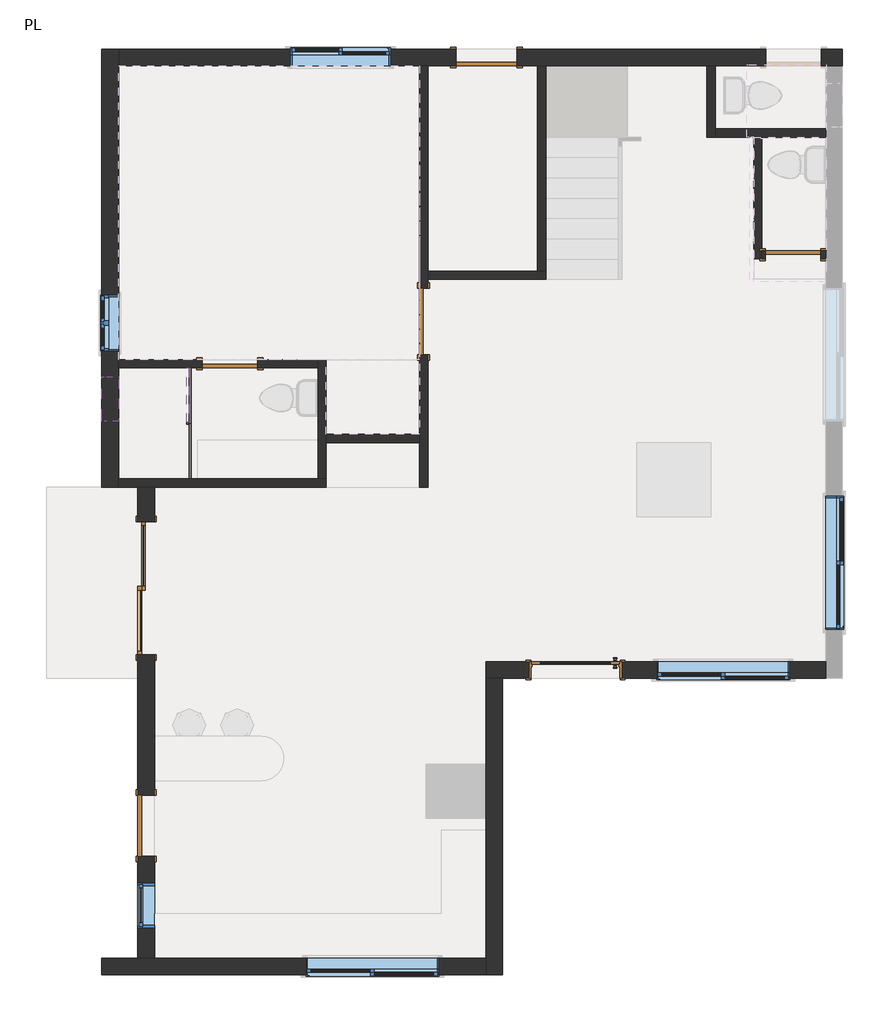
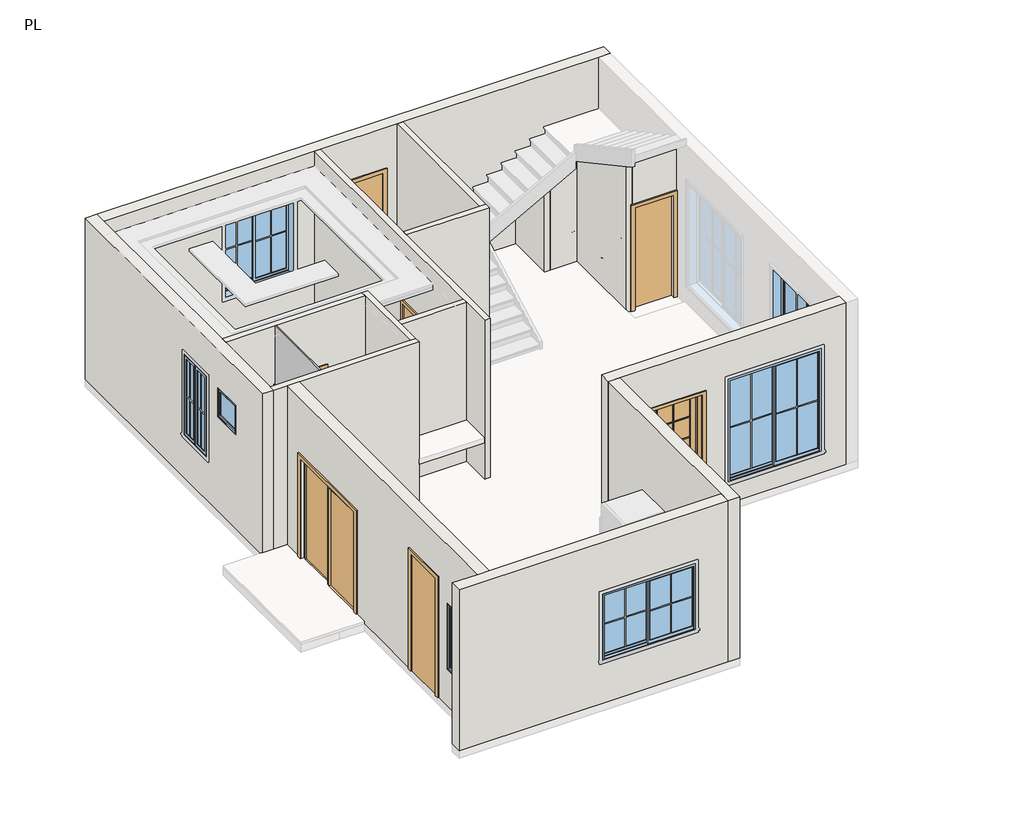
# One storey, part 1 of 2: 18 walls, 7 doors, 7 windows, 2 members, 2 plates.
"""IFC4 building model written with IfcOpenShell, lengths in millimetres."""

from ifc_helpers import new_model, si_unit, frame, origin, origin_with_axes, place, context, project, spatial, polyline, outline, extrude, faceted_brep, transform, mapped, element, save
from components import door_d4d75d1e, door_6ee39103, door_4b41b0c1, door_214872d5, door_78caadf7, door_5e62189b, member_12606fcf, member_8547658d, system_panel_glazed_13fc6ba1, system_panel_glazed_f04876f4, window_41ad1500, window_80340324, window_9dcce3b5, window_5810691a, window_sliding_double_6_x7_726fea71, window_sliding_double_6_x7_2_7e5eac46

model = new_model("IFC4")

# Units and contexts
model_context = context("Model", 3, world=origin())
ifc_project = project(units=[si_unit("LENGTHUNIT", "METRE", prefix="MILLI")], contexts=[model_context])

# Site, building, storey
site = spatial("IfcSite", under=ifc_project)
building = spatial("IfcBuilding", under=site)
storey = spatial("IfcBuildingStorey", under=building, Name="PL", Elevation=0.0)

# Doors
placement = place(None, origin())
door_shape = door_d4d75d1e(model_context)
element("IfcDoor", 1, ObjectType="Door-Double-Sliding : 72\" x 84\"", at=placement, inside=storey, context=model_context, shape_type="MappedRepresentation", body=[
    mapped(door_shape, transform((-13187.7002526, 4991.5628362, 0.0), x_axis=(0.0, 1.0, 0.0), y_axis=(-1.0, 0.0, 0.0), z_axis=(0.0, 0.0, 1.0))),
])
door_2_shape = door_6ee39103(model_context)
element("IfcDoor", 2, ObjectType="Door-Interior-Single-Full Glass-Wood : 48\" x 96\"", at=placement, inside=storey, context=model_context, shape_type="MappedRepresentation", body=[
    mapped(door_2_shape, transform((-7409.2002526, 3870.7877283, 0.0), x_axis=(-1.0, 0.0, 0.0), y_axis=(0.0, -1.0, 0.0), z_axis=(0.0, 0.0, 1.0))),
])
door_3_shape = door_4b41b0c1(model_context)
element("IfcDoor", 3, ObjectType="Single-Flush : 2'9\"X8'", at=placement, inside=storey, context=model_context, shape_type="MappedRepresentation", body=[
    mapped(door_3_shape, transform((-8634.7502526, 12287.7128362, 0.0), x_axis=(-1.0, 0.0, 0.0), y_axis=(0.0, -1.0, 0.0), z_axis=(0.0, 0.0, 1.0))),
])
element("IfcDoor", 4, ObjectType="Single-Flush : 2'9\"X8'", at=placement, inside=storey, context=model_context, shape_type="MappedRepresentation", body=[
    mapped(door_3_shape, transform((-13314.7002526, 1723.6940862, 0.0), x_axis=(0.0, 1.0, 0.0), y_axis=(-1.0, 0.0, 0.0), z_axis=(0.0, 0.0, 1.0))),
])
door_4_shape = door_214872d5(model_context)
element("IfcDoor", 5, ObjectType="Single-Flush : 30\" x 84\"", at=placement, inside=storey, context=model_context, shape_type="MappedRepresentation", body=[
    mapped(door_4_shape, transform((-4418.3502526, 9576.2628362, 0.0), x_axis=(1.0, 0.0, 0.0), y_axis=(0.0, 1.0, 0.0), z_axis=(0.0, 0.0, 1.0))),
])
door_5_shape = door_78caadf7(model_context)
element("IfcDoor", 6, ObjectType="Single-Flush : 30\" x 84\"", at=placement, inside=storey, context=model_context, shape_type="MappedRepresentation", body=[
    mapped(door_5_shape, transform((-12165.3502526, 8077.6628362, 0.0), x_axis=(1.0, 0.0, 0.0), y_axis=(0.0, 1.0, 0.0), z_axis=(0.0, 0.0, 1.0))),
])
door_6_shape = door_5e62189b(model_context)
element("IfcDoor", 7, ObjectType="Single-Flush : 36\" x 80\"", at=placement, inside=storey, context=model_context, shape_type="MappedRepresentation", body=[
    mapped(door_6_shape, transform((-9498.3502526, 8661.8628362, 0.0), x_axis=(0.0, -1.0, 0.0), y_axis=(1.0, 0.0, 0.0), z_axis=(0.0, 0.0, 1.0))),
])

# Members
member_shape = member_12606fcf(model_context)
element("IfcMember", 8, ObjectType="Rectangular Mullion : 1\" Square", at=placement, inside=storey, context=model_context, shape_type="MappedRepresentation", body=[
    mapped(member_shape, transform((-12743.285432, 7271.2128362, 2133.6), x_axis=(0.0, 0.0, 1.0), y_axis=(-1.0, 0.0, 0.0), z_axis=(0.0, -1.0, 0.0))),
])
member_2_shape = member_8547658d(model_context)
element("IfcMember", 9, ObjectType="Rectangular Mullion : 1\" Square", at=placement, inside=storey, context=model_context, shape_type="MappedRepresentation", body=[
    mapped(member_2_shape, transform((-12743.285432, 7258.5128362, 0.0), x_axis=(0.0, -1.0, 0.0), y_axis=(-1.0, 0.0, 0.0), z_axis=(0.0, 0.0, -1.0))),
])

# Plates
system_panel_glazed_shape = system_panel_glazed_13fc6ba1(model_context)
element("IfcPlate", 10, ObjectType="System Panel : Glazed", at=placement, inside=storey, context=model_context, shape_type="MappedRepresentation", body=[
    mapped(system_panel_glazed_shape, transform((-12743.285432, 7639.5128362, 0.0), x_axis=(0.0, -1.0, 0.0), y_axis=(1.0, 0.0, 0.0), z_axis=(0.0, 0.0, 1.0))),
])
system_panel_glazed_2_shape = system_panel_glazed_f04876f4(model_context)
element("IfcPlate", 11, ObjectType="System Panel : Glazed", at=placement, inside=storey, context=model_context, shape_type="MappedRepresentation", body=[
    mapped(system_panel_glazed_2_shape, transform((-12743.285432, 7258.5128362, 0.0), x_axis=(0.0, -1.0, 0.0), y_axis=(1.0, 0.0, 0.0), z_axis=(0.0, 0.0, 1.0))),
])

# Walls
element("IfcWall", 12, ObjectType="10\"", at=placement, inside=storey, context=model_context, shape_type="Brep", body=[
    faceted_brep([(-13924.3002526, 12402.0128362, 0.0), (-13924.3002526, 6382.2128362, 0.0), (-13924.3002526, 6382.2128362, 3352.8), (-13924.3002526, 12402.0128362, 3352.8), (-13924.3002526, 7899.8628362, 2565.4), (-13924.3002526, 7290.2628362, 2565.4), (-13924.3002526, 7290.2628362, 1955.8), (-13924.3002526, 7899.8628362, 1955.8), (-13924.3002526, 9017.4628362, 2590.8), (-13924.3002526, 8255.4628362, 2590.8), (-13924.3002526, 8255.4628362, 914.4), (-13924.3002526, 9017.4628362, 914.4), (-13695.7002526, 12402.0128362, 0.0), (-13695.7002526, 12402.0128362, 3352.8), (-13695.7002526, 12173.4128362, 3352.8), (-13695.7002526, 8134.8128362, 3352.8), (-13695.7002526, 8020.5128362, 3352.8), (-13695.7002526, 6496.5128362, 3352.8), (-13695.7002526, 6382.2128362, 3352.8), (-13695.7002526, 6382.2128362, 0.0), (-13695.7002526, 6496.5128362, 0.0), (-13695.7002526, 8020.5128362, 0.0), (-13695.7002526, 8134.8128362, 0.0), (-13695.7002526, 12173.4128362, 0.0), (-13695.7002526, 7899.8628362, 2565.4), (-13695.7002526, 7899.8628362, 1955.8), (-13695.7002526, 7290.2628362, 1955.8), (-13695.7002526, 7290.2628362, 2565.4), (-13695.7002526, 9017.4628362, 2590.8), (-13695.7002526, 9017.4628362, 914.4), (-13695.7002526, 8255.4628362, 914.4), (-13695.7002526, 8255.4628362, 2590.8)], [[[0, 1, 2, 3], [4, 5, 6, 7], [8, 9, 10, 11]], [[12, 13, 14, 15, 16, 17, 18, 19, 20, 21, 22, 23], [24, 25, 26, 27], [28, 29, 30, 31]], [[1, 0, 12, 23, 22, 21, 20, 19]], [[3, 2, 18, 17, 16, 15, 14, 13]], [[2, 1, 19, 18]], [[0, 3, 13, 12]], [[25, 24, 4, 7]], [[26, 25, 7, 6]], [[27, 26, 6, 5]], [[24, 27, 5, 4]], [[29, 28, 8, 11]], [[30, 29, 11, 10]], [[31, 30, 10, 9]], [[28, 31, 9, 8]]]),
])
element("IfcWall", 13, ObjectType="10\"", at=placement, inside=storey, context=model_context, shape_type="Brep", body=[
    faceted_brep([(-13695.7002526, 12173.4128362, 0.0), (-9555.5002526, 12173.4128362, 0.0), (-9441.2002526, 12173.4128362, 0.0), (-9053.8502526, 12173.4128362, 0.0), (-9053.8502526, 12173.4128362, 2438.4), (-8215.6502526, 12173.4128362, 2438.4), (-8215.6502526, 12173.4128362, 0.0), (-7929.9002526, 12173.4128362, 0.0), (-7815.6002526, 12173.4128362, 0.0), (-5599.4131221, 12173.4128362, 0.0), (-5485.1131221, 12173.4128362, 0.0), (-4793.0002526, 12173.4128362, 0.0), (-4793.0002526, 12173.4128362, 2133.6), (-4031.0002526, 12173.4128362, 2133.6), (-4031.0002526, 12173.4128362, 0.0), (-3967.5002526, 12173.4128362, 0.0), (-3738.9002526, 12173.4128362, 0.0), (-3738.9002526, 12173.4128362, 3352.8), (-3967.5002526, 12173.4128362, 3352.8), (-7815.6002526, 12173.4128362, 3352.8), (-7929.9002526, 12173.4128362, 3352.8), (-9441.2002526, 12173.4128362, 3352.8), (-9555.5002526, 12173.4128362, 3352.8), (-13695.7002526, 12173.4128362, 3352.8), (-9955.5502526, 12173.4128362, 2590.8), (-9955.5502526, 12173.4128362, 914.4), (-11327.1502526, 12173.4128362, 914.4), (-11327.1502526, 12173.4128362, 2590.8), (-9053.8502526, 12402.0128362, 2438.4), (-9053.8502526, 12402.0128362, 0.0), (-13695.7002526, 12402.0128362, 0.0), (-13695.7002526, 12402.0128362, 3352.8), (-3738.9002526, 12402.0128362, 3352.8), (-3738.9002526, 12402.0128362, 0.0), (-4031.0002526, 12402.0128362, 0.0), (-4031.0002526, 12402.0128362, 2133.6), (-4793.0002526, 12402.0128362, 2133.6), (-4793.0002526, 12402.0128362, 0.0), (-8215.6502526, 12402.0128362, 0.0), (-8215.6502526, 12402.0128362, 2438.4), (-9955.5502526, 12402.0128362, 2590.8), (-11327.1502526, 12402.0128362, 2590.8), (-11327.1502526, 12402.0128362, 914.4), (-9955.5502526, 12402.0128362, 914.4)], [[[0, 1, 2, 3, 4, 5, 6, 7, 8, 9, 10, 11, 12, 13, 14, 15, 16, 17, 18, 19, 20, 21, 22, 23], [24, 25, 26, 27]], [[28, 29, 30, 31, 32, 33, 34, 35, 36, 37, 38, 39], [40, 41, 42, 43]], [[16, 15, 14, 34, 33]], [[38, 37, 11, 10, 9, 8, 7, 6]], [[30, 29, 3, 2, 1, 0]], [[23, 22, 21, 20, 19, 18, 17, 32, 31]], [[0, 23, 31, 30]], [[17, 16, 33, 32]], [[35, 34, 14, 13]], [[36, 35, 13, 12]], [[37, 36, 12, 11]], [[4, 3, 29, 28]], [[5, 4, 28, 39]], [[6, 5, 39, 38]], [[25, 24, 40, 43]], [[26, 25, 43, 42]], [[27, 26, 42, 41]], [[24, 27, 41, 40]]]),
])
element("IfcWall", 14, ObjectType="10\"", at=placement, inside=storey, context=model_context, shape_type="Brep", body=[
    faceted_brep([(-8641.1002526, 3981.9127283, 3352.8), (-3967.5002526, 3981.9127283, 3352.8), (-3967.5002526, 3981.9127283, 0.0), (-6774.2002526, 3981.9127283, 0.0), (-6774.2002526, 3981.9127283, 2463.8), (-8044.2002526, 3981.9127283, 2463.8), (-8044.2002526, 3981.9127283, 0.0), (-8641.1002526, 3981.9127283, 0.0), (-6291.6002526, 3981.9127283, 2590.8), (-6291.6002526, 3981.9127283, 457.2), (-4462.8002526, 3981.9127283, 457.2), (-4462.8002526, 3981.9127283, 2590.8), (-3967.5002526, 3753.3127283, 3352.8), (-8412.5002526, 3753.3127283, 3352.8), (-8641.1002526, 3753.3127283, 3352.8), (-8641.1002526, 3753.3127283, 0.0), (-8412.5002526, 3753.3127283, 0.0), (-8044.2002526, 3753.3127283, 0.0), (-8044.2002526, 3753.3127283, 2463.8), (-6774.2002526, 3753.3127283, 2463.8), (-6774.2002526, 3753.3127283, 0.0), (-3967.5002526, 3753.3127283, 0.0), (-6291.6002526, 3753.3127283, 2590.8), (-4462.8002526, 3753.3127283, 2590.8), (-4462.8002526, 3753.3127283, 457.2), (-6291.6002526, 3753.3127283, 457.2)], [[[0, 1, 2, 3, 4, 5, 6, 7], [8, 9, 10, 11]], [[12, 13, 14, 15, 16, 17, 18, 19, 20, 21], [22, 23, 24, 25]], [[2, 21, 20, 3]], [[15, 7, 6, 17, 16]], [[1, 0, 14, 13, 12]], [[2, 1, 12, 21]], [[0, 7, 15, 14]], [[5, 18, 17, 6]], [[18, 5, 4, 19]], [[19, 4, 3, 20]], [[9, 8, 22, 25]], [[10, 9, 25, 24]], [[11, 10, 24, 23]], [[8, 11, 23, 22]]]),
])
element("IfcWall", 15, ObjectType="10\"", at=placement, inside=storey, context=model_context, shape_type="Brep", body=[
    faceted_brep([(-8641.1002526, 3753.3127283, 0.0), (-8641.1002526, -92.4059138, 0.0), (-8641.1002526, -321.0059138, 0.0), (-8641.1002526, -321.0059138, 3352.8), (-8641.1002526, -92.4059138, 3352.8), (-8641.1002526, 3753.3127283, 3352.8), (-8412.5002526, 3753.3127283, 0.0), (-8412.5002526, 3753.3127283, 3352.8), (-8412.5002526, -321.0059138, 3352.8), (-8412.5002526, -321.0059138, 0.0)], [[[0, 1, 2, 3, 4, 5]], [[6, 7, 8, 9]], [[2, 1, 0, 6, 9]], [[5, 4, 3, 8, 7]], [[0, 5, 7, 6]], [[3, 2, 9, 8]]]),
])
element("IfcWall", 16, ObjectType="10\"", at=placement, inside=storey, context=model_context, shape_type="Brep", body=[
    faceted_brep([(-8641.1002526, -92.4059138, 0.0), (-13200.4002526, -92.4059138, 0.0), (-13429.0002526, -92.4059138, 0.0), (-13925.8877526, -92.4059138, 0.0), (-13925.8877526, -92.4059138, 3352.8), (-13429.0002526, -92.4059138, 3352.8), (-13200.4002526, -92.4059138, 3352.8), (-8641.1002526, -92.4059138, 3352.8), (-11117.6002526, -92.4059138, 2286.0), (-11117.6002526, -92.4059138, 914.4), (-9288.8002526, -92.4059138, 914.4), (-9288.8002526, -92.4059138, 2286.0), (-8641.1002526, -321.0059138, 0.0), (-8641.1002526, -321.0059138, 3352.8), (-13925.8877526, -321.0059138, 3352.8), (-13925.8877526, -321.0059138, 0.0), (-11117.6002526, -321.0059138, 2286.0), (-9288.8002526, -321.0059138, 2286.0), (-9288.8002526, -321.0059138, 914.4), (-11117.6002526, -321.0059138, 914.4)], [[[0, 1, 2, 3, 4, 5, 6, 7], [8, 9, 10, 11]], [[12, 13, 14, 15], [16, 17, 18, 19]], [[3, 2, 1, 0, 12, 15]], [[4, 3, 15, 14]], [[7, 6, 5, 4, 14, 13]], [[0, 7, 13, 12]], [[9, 8, 16, 19]], [[10, 9, 19, 18]], [[11, 10, 18, 17]], [[8, 11, 17, 16]]]),
])
element("IfcWall", 17, ObjectType="10\"", at=placement, inside=storey, context=model_context, shape_type="SweptSolid", body=[
    extrude(outline(polyline([(4077.1628362, 0.0), (2142.7940862, 0.0), (2142.7940862, 2438.4), (1304.5940862, 2438.4), (1304.5940862, 0.0), (-92.4059138, 0.0), (-92.4059138, 3352.8), (6382.2128362, 3352.8), (6382.2128362, 0.0), (5905.9628362, 0.0), (5905.9628362, 2133.6), (4077.1628362, 2133.6), (4077.1628362, 0.0)]), holes=[polyline([(936.2940862, 2133.6), (326.6940862, 2133.6), (326.6940862, 762.0), (936.2940862, 762.0), (936.2940862, 2133.6)])]), frame((-13429.0002526, 0.0, 0.0), z_axis=(1.0, 0.0, 0.0), x_axis=(0.0, 1.0, 0.0)), (0.0, 0.0, 1.0), 228.6),
])
element("IfcWall", 18, ObjectType="5\"", at=placement, inside=storey, context=model_context, shape_type="Brep", body=[
    faceted_brep([(-13695.7002526, 6382.2128362, 0.0), (-13429.0002526, 6382.2128362, 0.0), (-13200.4002526, 6382.2128362, 0.0), (-10838.2002526, 6382.2128362, 0.0), (-10838.2002526, 6382.2128362, 3352.8), (-13200.4002526, 6382.2128362, 3352.8), (-13429.0002526, 6382.2128362, 3352.8), (-13695.7002526, 6382.2128362, 3352.8), (-13695.7002526, 6496.5128362, 0.0), (-13695.7002526, 6496.5128362, 3352.8), (-10952.5002526, 6496.5128362, 3352.8), (-10838.2002526, 6496.5128362, 3352.8), (-10838.2002526, 6496.5128362, 0.0), (-10952.5002526, 6496.5128362, 0.0)], [[[0, 1, 2, 3, 4, 5, 6, 7]], [[8, 9, 10, 11, 12, 13]], [[3, 2, 1, 0, 8, 13, 12]], [[7, 6, 5, 4, 11, 10, 9]], [[0, 7, 9, 8]], [[4, 3, 12, 11]]]),
])
element("IfcWall", 19, ObjectType="5\"", at=placement, inside=storey, context=model_context, shape_type="Brep", body=[
    faceted_brep([(-10838.2002526, 6496.5128362, 0.0), (-10838.2002526, 6991.8128362, 0.0), (-10838.2002526, 7106.1128362, 0.0), (-10838.2002526, 8134.8128362, 0.0), (-10838.2002526, 8134.8128362, 3352.8), (-10838.2002526, 7106.1128362, 3352.8), (-10838.2002526, 6991.8128362, 3352.8), (-10838.2002526, 6496.5128362, 3352.8), (-10952.5002526, 6496.5128362, 0.0), (-10952.5002526, 6496.5128362, 3352.8), (-10952.5002526, 8020.5128362, 3352.8), (-10952.5002526, 8134.8128362, 3352.8), (-10952.5002526, 8134.8128362, 0.0), (-10952.5002526, 8020.5128362, 0.0)], [[[0, 1, 2, 3, 4, 5, 6, 7]], [[8, 9, 10, 11, 12, 13]], [[3, 2, 1, 0, 8, 13, 12]], [[7, 6, 5, 4, 11, 10, 9]], [[0, 7, 9, 8]], [[4, 3, 12, 11]]]),
])
element("IfcWall", 20, ObjectType="5\"", at=placement, inside=storey, context=model_context, shape_type="SweptSolid", body=[
    extrude(outline(polyline([(2133.6, -11784.3502526), (0.0, -11784.3502526), (0.0, -10952.5002526), (3352.8, -10952.5002526), (3352.8, -13695.7002526), (0.0, -13695.7002526), (0.0, -12546.3502526), (2133.6, -12546.3502526), (2133.6, -11784.3502526)])), frame((0.0, 8020.5128362, 0.0), z_axis=(0.0, 1.0, 0.0), x_axis=(0.0, 0.0, 1.0)), (0.0, 0.0, 1.0), 114.3),
])
element("IfcWall", 21, ObjectType="5\"", at=placement, inside=storey, context=model_context, shape_type="SweptSolid", body=[
    extrude(outline(polyline([(-9555.5002526, 6991.8128362), (-10838.2002526, 6991.8128362), (-10838.2002526, 7106.1128362), (-9555.5002526, 7106.1128362), (-9555.5002526, 6991.8128362)])), origin_with_axes(), (0.0, 0.0, 1.0), 3352.8),
])
element("IfcWall", 22, ObjectType="5\"", at=placement, inside=storey, context=model_context, shape_type="Brep", body=[
    faceted_brep([(-9441.2002526, 6382.2128362, 0.0), (-9441.2002526, 8204.6628362, 0.0), (-9441.2002526, 8204.6628362, 2032.0), (-9441.2002526, 9119.0628362, 2032.0), (-9441.2002526, 9119.0628362, 0.0), (-9441.2002526, 9239.7128362, 0.0), (-9441.2002526, 9354.0128362, 0.0), (-9441.2002526, 12173.4128362, 0.0), (-9441.2002526, 12173.4128362, 3352.8), (-9441.2002526, 9354.0128362, 3352.8), (-9441.2002526, 9239.7128362, 3352.8), (-9441.2002526, 6382.2128362, 3352.8), (-9555.5002526, 8204.6628362, 2032.0), (-9555.5002526, 8204.6628362, 0.0), (-9555.5002526, 7106.1128362, 0.0), (-9555.5002526, 6991.8128362, 0.0), (-9555.5002526, 6382.2128362, 0.0), (-9555.5002526, 6382.2128362, 3352.8), (-9555.5002526, 6991.8128362, 3352.8), (-9555.5002526, 7106.1128362, 3352.8), (-9555.5002526, 12173.4128362, 3352.8), (-9555.5002526, 12173.4128362, 0.0), (-9555.5002526, 9119.0628362, 0.0), (-9555.5002526, 9119.0628362, 2032.0)], [[[0, 1, 2, 3, 4, 5, 6, 7, 8, 9, 10, 11]], [[12, 13, 14, 15, 16, 17, 18, 19, 20, 21, 22, 23]], [[22, 21, 7, 6, 5, 4]], [[16, 15, 14, 13, 1, 0]], [[11, 10, 9, 8, 20, 19, 18, 17]], [[0, 11, 17, 16]], [[8, 7, 21, 20]], [[2, 1, 13, 12]], [[3, 2, 12, 23]], [[4, 3, 23, 22]]]),
])
element("IfcWall", 23, ObjectType="5\"", at=placement, inside=storey, context=model_context, shape_type="Brep", body=[
    faceted_brep([(-9441.2002526, 9239.7128362, 0.0), (-7815.6002526, 9239.7128362, 0.0), (-7815.6002526, 9239.7128362, 3352.8), (-9441.2002526, 9239.7128362, 3352.8), (-9441.2002526, 9354.0128362, 0.0), (-9441.2002526, 9354.0128362, 3352.8), (-7929.9002526, 9354.0128362, 3352.8), (-7815.6002526, 9354.0128362, 3352.8), (-7815.6002526, 9354.0128362, 0.0), (-7929.9002526, 9354.0128362, 0.0)], [[[0, 1, 2, 3]], [[4, 5, 6, 7, 8, 9]], [[1, 0, 4, 9, 8]], [[3, 2, 7, 6, 5]], [[0, 3, 5, 4]], [[2, 1, 8, 7]]]),
])
element("IfcWall", 24, ObjectType="5\"", at=placement, inside=storey, context=model_context, shape_type="SweptSolid", body=[
    extrude(outline(polyline([(-7815.6002526, 12173.4128362), (-7815.6002526, 9354.0128362), (-7929.9002526, 9354.0128362), (-7929.9002526, 12173.4128362), (-7815.6002526, 12173.4128362)])), origin_with_axes(), (0.0, 0.0, 1.0), 3352.8),
])
element("IfcWall", 25, ObjectType="5\"", at=placement, inside=storey, context=model_context, shape_type="Brep", body=[
    faceted_brep([(-5599.4131221, 12173.4128362, 0.0), (-5599.4131221, 11195.5128362, 0.0), (-5599.4131221, 11195.5128362, 1720.85), (-5599.4131221, 12173.4128362, 1720.85), (-5485.1131221, 12173.4128362, 0.0), (-5485.1131221, 12173.4128362, 1720.85), (-5485.1131221, 11195.5128362, 1720.85), (-5485.1131221, 11195.5128362, 0.0), (-5485.1131221, 11309.8128362, 0.0)], [[[0, 1, 2, 3]], [[4, 5, 6, 7, 8]], [[0, 3, 5, 4]], [[2, 1, 7, 6]], [[1, 0, 4, 8, 7]], [[3, 2, 6, 5]]]),
])
element("IfcWall", 26, ObjectType="5\"", at=placement, inside=storey, context=model_context, shape_type="Brep", body=[
    faceted_brep([(-5485.1131221, 11195.5128362, 0.0), (-4958.1002526, 11195.5128362, 0.0), (-4843.8002526, 11195.5128362, 0.0), (-3967.5002526, 11195.5128362, 0.0), (-3967.5002526, 11195.5128362, 2057.4), (-4935.5581325, 11195.5128362, 2057.4), (-5485.1131221, 11195.5128362, 1757.642733), (-5485.1131221, 11195.5128362, 1720.85), (-5485.1131221, 11309.8128362, 0.0), (-5485.1131221, 11309.8128362, 1757.642733), (-4935.5581325, 11309.8128362, 2057.4), (-3967.5002526, 11309.8128362, 2057.4), (-3967.5002526, 11309.8128362, 0.0)], [[[0, 1, 2, 3, 4, 5, 6, 7]], [[8, 9, 10, 11, 12]], [[0, 7, 6, 9, 8]], [[4, 3, 12, 11]], [[3, 2, 1, 0, 8, 12]], [[5, 4, 11, 10]], [[6, 5, 10, 9]]]),
])
element("IfcWall", 27, ObjectType="5\"", at=placement, inside=storey, context=model_context, shape_type="Brep", body=[
    faceted_brep([(-4958.1002526, 11195.5128362, 0.0), (-4958.1002526, 9519.1128362, 0.0), (-4958.1002526, 9519.1128362, 3059.9497528), (-4958.1002526, 11195.5128362, 2145.5497528), (-4843.8002526, 11195.5128362, 0.0), (-4843.8002526, 11195.5128362, 2145.5497528), (-4843.8002526, 9519.1128362, 3059.9497528), (-4843.8002526, 9519.1128362, 0.0), (-4843.8002526, 9633.4128362, 0.0)], [[[0, 1, 2, 3]], [[4, 5, 6, 7, 8]], [[0, 3, 5, 4]], [[2, 1, 7, 6]], [[1, 0, 4, 8, 7]], [[3, 2, 6, 5]]]),
])
element("IfcWall", 28, ObjectType="5\"", at=placement, inside=storey, context=model_context, shape_type="Brep", body=[
    faceted_brep([(-4037.3502526, 9519.1128362, 2133.6), (-4037.3502526, 9519.1128362, 0.0), (-3967.5002526, 9519.1128362, 0.0), (-3967.5002526, 9519.1128362, 3149.6), (-4843.8002526, 9519.1128362, 3149.6), (-4843.8002526, 9519.1128362, 3059.9497528), (-4843.8002526, 9519.1128362, 0.0), (-4799.3502526, 9519.1128362, 0.0), (-4799.3502526, 9519.1128362, 2133.6), (-3967.5002526, 9633.4128362, 0.0), (-4037.3502526, 9633.4128362, 0.0), (-4037.3502526, 9633.4128362, 2133.6), (-4799.3502526, 9633.4128362, 2133.6), (-4799.3502526, 9633.4128362, 0.0), (-4843.8002526, 9633.4128362, 0.0), (-4843.8002526, 9633.4128362, 3149.6), (-3967.5002526, 9633.4128362, 3149.6)], [[[0, 1, 2, 3, 4, 5, 6, 7, 8]], [[9, 10, 11, 12, 13, 14, 15, 16]], [[7, 6, 14, 13]], [[2, 1, 10, 9]], [[4, 3, 16, 15]], [[6, 5, 4, 15, 14]], [[3, 2, 9, 16]], [[11, 10, 1, 0]], [[12, 11, 0, 8]], [[13, 12, 8, 7]]]),
])
element("IfcWall", 29, ObjectType="5\"", at=placement, inside=storey, context=model_context, shape_type="SweptSolid", body=[
    extrude(outline(polyline([(-11841.5002526, 2345.9940862), (-11841.5002526, 2955.5940862), (-11727.2002526, 2955.5940862), (-11727.2002526, 2345.9940862), (-11841.5002526, 2345.9940862)])), origin_with_axes(), (0.0, 0.0, 1.0), 914.4),
])

# Windows
window_shape = window_41ad1500(model_context)
element("IfcWindow", 30, ObjectType="Fixed : 2'-0\" X 4'-6\"", at=placement, inside=storey, context=model_context, shape_type="MappedRepresentation", body=[
    mapped(window_shape, transform((-13314.7002526, 669.5940862, 0.0), x_axis=(0.0, 1.0, 0.0), y_axis=(-1.0, 0.0, 0.0), z_axis=(0.0, 0.0, 1.0))),
])
window_2_shape = window_80340324(model_context)
element("IfcWindow", 31, ObjectType="Fixed : 24\" x 24\"", at=placement, inside=storey, context=model_context, shape_type="MappedRepresentation", body=[
    mapped(window_2_shape, transform((-13810.0002526, 7633.1628362, 1041.4), x_axis=(0.0, 1.0, 0.0), y_axis=(-1.0, 0.0, 0.0), z_axis=(0.0, 0.0, 1.0))),
])
window_3_shape = window_9dcce3b5(model_context)
element("IfcWindow", 32, ObjectType="Window-Casement-Double : 2'-6\" X 5'-6\"", at=placement, inside=storey, context=model_context, shape_type="MappedRepresentation", body=[
    mapped(window_3_shape, transform((-13810.0002526, 8636.4628362, 0.0), x_axis=(0.0, 1.0, 0.0), y_axis=(-1.0, 0.0, 0.0), z_axis=(0.0, 0.0, 1.0))),
])
window_4_shape = window_5810691a(model_context)
element("IfcWindow", 33, ObjectType="Window-Sliding-Double : 54\" x 66\"", at=placement, inside=storey, context=model_context, shape_type="MappedRepresentation", body=[
    mapped(window_4_shape, transform((-10641.3502526, 12291.5228362, 0.0), x_axis=(1.0, 0.0, 0.0), y_axis=(0.0, 1.0, 0.0), z_axis=(0.0, 0.0, 1.0))),
])
window_sliding_double_6_x7_shape = window_sliding_double_6_x7_726fea71(model_context)
element("IfcWindow", 34, ObjectType="Window-Sliding-Double : 6'X7'", at=placement, inside=storey, context=model_context, shape_type="MappedRepresentation", body=[
    mapped(window_sliding_double_6_x7_shape, transform((-3849.3902526, 5340.8127283, -457.2), x_axis=(0.0, -1.0, 0.0), y_axis=(1.0, 0.0, 0.0), z_axis=(0.0, 0.0, 1.0))),
])
element("IfcWindow", 35, ObjectType="Window-Sliding-Double : 6'X7'", at=placement, inside=storey, context=model_context, shape_type="MappedRepresentation", body=[
    mapped(window_sliding_double_6_x7_shape, transform((-5377.2002526, 3863.8027283, -457.2), x_axis=(-1.0, 0.0, 0.0), y_axis=(0.0, -1.0, 0.0), z_axis=(0.0, 0.0, 1.0))),
])
window_sliding_double_6_x7_2_shape = window_sliding_double_6_x7_2_7e5eac46(model_context)
element("IfcWindow", 36, ObjectType="Window-Sliding-Double : 6'X7' 2", at=placement, inside=storey, context=model_context, shape_type="MappedRepresentation", body=[
    mapped(window_sliding_double_6_x7_2_shape, transform((-10203.2002526, -210.5159138, 0.0), x_axis=(-1.0, 0.0, 0.0), y_axis=(0.0, -1.0, 0.0), z_axis=(0.0, 0.0, 1.0))),
])

save(model, "model.ifc")

# Revit data of these elements
# Type "Door-Double-Sliding : 72\" x 84\""
#   Type Mark = "10"
#   Construction Type Id = "opn-d45"
#   Assembly Code = "C1020"
#   Analytic Construction = "Wood frame, double glass door "
#   Thickness = 0' - 2"
#   Thermal Resistance (R) = 1.8150 (h·ft²·°F)/BTU
#   Heat Transfer Coefficient (U) = 0.5510 BTU/(h·ft²·°F)
#   Height = 7' - 0"
#   Rail Width = 0' - 2"
#   Stiles = 0' - 2"
#   Trim Projection Ext = 0' - 1"
#   Trim Projection Int = 0' - 1"
#   Trim Width = 0' - 3"
#   Width = 6' - 0"
#   Define Thermal Properties by = 1
#   Glazing = Glass
#   Panel Material = Wood - Birch - Solid Stained Light Low Gloss
#   Trim Material = Paint - Sienna
#   Visual Light Transmittance = 0
#   Solar Heat Gain Coefficient = 0
#   Function = (empty or 0)
#   Wall Closure = (empty or 0)
# Type "Door-Interior-Single-Full Glass-Wood : 48\" x 96\""
#   Type Mark = "8"
#   Assembly Code = "C1020300"
#   Analytic Construction = "Wood frame with single clear glass"
#   Top Rail = 0' - 4 11/16"
#   Thickness = 0' - 1 3/8"
#   Thermal Resistance (R) = 1.0102 (h·ft²·°F)/BTU
#   Swing Angle [instance default] = 90.00°
#   Stiles = 0' - 4 3/4"
#   Rough Width = 4' - 2"
#   Rough Height = 8' - 1"
#   Height = 8' - 0"
#   Width = 4' - 0"
#   Heat Transfer Coefficient (U) = 0.9900 BTU/(h·ft²·°F)
#   Bottom Rail = 0' - 9 1/8"
#   Show Grill [instance default] = yes
#   Trim Material = Cherry
#   Panel Material = Cherry
#   Frame Material = Cherry
#   Door Handle Material = Aluminum
#   Visual Light Transmittance = 0
#   Solar Heat Gain Coefficient = 0
#   Wall Closure = (empty or 0)
#   Function = (empty or 0)
# Type "Single-Flush : 2'9\"X8'"
#   Type Mark = "9"
#   Construction Type Id = "MDOOR"
#   Assembly Code = "C1020"
#   Analytic Construction = "Metal"
#   Thickness = 0' - 2"
#   Heat Transfer Coefficient (U) = 0.651978 BTU/(h·ft²·°F)
#   Height = 8' - 0"
#   Trim Projection Ext = 0' - 1"
#   Trim Projection Int = 0' - 1"
#   Trim Width = 0' - 3"
#   Width = 2' - 9"
#   Define Thermal Properties by = 1
#   Door Material = Door - Panel
#   Frame Material = Door - Frame
#   Visual Light Transmittance = 0
#   Solar Heat Gain Coefficient = 0
#   Function = (empty or 0)
#   Wall Closure = (empty or 0)
# Type "Single-Flush : 30\" x 84\""
#   Type Mark = "4"
#   Construction Type Id = "MDOOR"
#   Assembly Code = "C1020"
#   Analytic Construction = "Metal"
#   Thickness = 0' - 2"
#   Heat Transfer Coefficient (U) = 0.651978 BTU/(h·ft²·°F)
#   Height = 7' - 0"
#   Trim Projection Ext = 0' - 1"
#   Trim Projection Int = 0' - 1"
#   Trim Width = 0' - 3"
#   Width = 2' - 6"
#   Define Thermal Properties by = 1
#   Define Thermal Properties by = 1
#   Door Material = Door - Panel
#   Frame Material = Door - Frame
#   Visual Light Transmittance = 0
#   Solar Heat Gain Coefficient = 0
#   Function = (empty or 0)
#   Wall Closure = (empty or 0)
# Type "Single-Flush : 36\" x 80\""
#   Type Mark = "6"
#   Construction Type Id = "MDOOR"
#   Assembly Code = "C1020"
#   Analytic Construction = "Metal"
#   Thickness = 0' - 2"
#   Heat Transfer Coefficient (U) = 0.651978 BTU/(h·ft²·°F)
#   Height = 6' - 8"
#   Trim Projection Ext = 0' - 1"
#   Trim Projection Int = 0' - 1"
#   Trim Width = 0' - 3"
#   Width = 3' - 0"
#   Define Thermal Properties by = 1
#   Define Thermal Properties by = 1
#   Door Material = Door - Panel
#   Frame Material = Door - Frame
#   Visual Light Transmittance = 0
#   Solar Heat Gain Coefficient = 0
#   Function = (empty or 0)
#   Wall Closure = (empty or 0)
# Type "Rectangular Mullion : 1\" Square"
#   built-in parameter 1007304 = 0.0833333 (stored number, unit not read)
#   built-in parameter 1007301 = 0.0416667 (stored number, unit not read)
#   built-in parameter 1007300 = 0.0416667 (stored number, unit not read)
# Type "System Panel : Glazed"
#   Construction Type Id = "GSP4R"
#   Analytic Construction = "1/8 in Pilkington single glazing"
#   Visual Light Transmittance = 0.9
#   Solar Heat Gain Coefficient = 0.86
#   Heat Transfer Coefficient (U) = 1.18115 BTU/(h·ft²·°F)
#   Define Thermal Properties by = 1
# Type "10\""
#   Assembly Code = "B2010"
#   Layers, outside or top first: 0' - 9" "Gypsum Wall Board" (function 1)
# Type "5\""
#   Assembly Code = "B2010"
#   Layers, outside or top first: 0' - 4 1/2" "Gypsum Wall Board" (function 1)
# Type "Fixed : 2'-0\" X 4'-6\""
#   Type Mark = "22"
#   Construction Type Id = "GSP4R"
#   Assembly Code = "B2020100"
#   Analytic Construction = "1/8 in Pilkington single glazing"
#   Visual Light Transmittance = 0.9
#   Solar Heat Gain Coefficient = 0.78
#   Heat Transfer Coefficient (U) = 0.6496 BTU/(h·ft²·°F)
#   Height = 4' - 6"
#   Default Sill Height = 2' - 6"
#   Width = 2' - 0"
#   Window Inset = 0' - 0 3/4"
#   Define Thermal Properties by = 1
#   Glass Pane Material = Glass
#   Sash Material = Sash
#   Wall Closure = (empty or 0)
# Type "Fixed : 24\" x 24\""
#   Type Mark = "3"
#   Construction Type Id = "GSP4R"
#   Assembly Code = "B2020100"
#   Analytic Construction = "1/8 in Pilkington single glazing"
#   Visual Light Transmittance = 0.9
#   Solar Heat Gain Coefficient = 0.78
#   Heat Transfer Coefficient (U) = 0.6496 BTU/(h·ft²·°F)
#   Height = 2' - 0"
#   Default Sill Height = 3' - 0"
#   Width = 2' - 0"
#   Window Inset = 0' - 0 3/4"
#   Define Thermal Properties by = 1
#   Define Thermal Properties by = 1
#   Glass Pane Material = Glass
#   Sash Material = Sash
#   Wall Closure = (empty or 0)
# Type "Window-Casement-Double : 2'-6\" X 5'-6\""
#   Type Mark = "21"
#   Fire Rating = "0.5h"
#   Assembly Code = "B2020100"
#   Analytic Construction = "Double glazing - domestic"
#   Frame Extension [instance default] = 0' - 0 1/4"
#   Window Inset [instance default] = 0' - 0"
#   Wall Thickness [instance default] = 0' - 6"
#   Interior Wall Closure [instance default] = 0' - 2 1/4"
#   Half Width = 1' - 3"
#   Visual Light Transmittance = 0.81
#   Thermal Resistance (R) = 1.8146 (h·ft²·°F)/BTU
#   Solar Heat Gain Coefficient = 0.76
#   Rough Width = 2' - 6 1/2"
#   Rough Height = 5' - 6 1/2"
#   Height = 5' - 6"
#   Heat Transfer Coefficient (U) = 0.5511 BTU/(h·ft²·°F)
#   Exterior Wall Closure [instance default] = 0' - 1 1/4"
#   Extension Jamb [instance default] = 0' - 2 1/4"
#   Default Sill Height = 3' - 0"
#   Width = 2' - 6"
#   Muntin Visibility = yes
#   Interior Trim Visibility [instance default] = yes
#   Exterior Trim Visibility [instance default] = yes
#   Extension Jamb Visibility [instance default] = yes
#   Interior Trim Material = Wood - Stained
#   Muntin Pattern = Muntin Pattern_2x2 : Muntin Pattern_2x2
#   Interior Trim = Trim-Window-Interior-Flat : Picture Frame
#   Interior Frame Material = Wood - Stained
#   Glass Panel Material = Glass
#   Exterior Trim Material = Clad - White
#   Exterior Trim = Trim-Window-Exterior-Flat : with Sill
#   Exterior Frame Material = Clad - White
#   Wall Closure = (empty or 0)
# Type "Window-Sliding-Double : 54\" x 66\""
#   Type Mark = "20"
#   Fire Rating = "0.5h"
#   Assembly Code = "B2020100"
#   Analytic Construction = "Double glazing - domestic"
#   Window Inset [instance default] = 0' - 0"
#   Wall Thickness [instance default] = 0' - 6"
#   Visual Light Transmittance = 0.81
#   Thermal Resistance (R) = 1.8146 (h·ft²·°F)/BTU
#   Solar Heat Gain Coefficient = 0.76
#   Muntin Width = 1' - 11 5/8"
#   Muntin Height = 5' - 0 1/4"
#   Interior Wall Closure [instance default] = 0' - 2 3/4"
#   Heat Transfer Coefficient (U) = 0.5511 BTU/(h·ft²·°F)
#   Frame Extension [instance default] = 0' - 0 1/4"
#   Exterior Wall Closure [instance default] = 0' - 1 1/4"
#   Rough Width = 4' - 6 1/2"
#   Rough Height = 5' - 6 1/2"
#   Height = 5' - 6"
#   Extension Jamb [instance default] = 0' - 2 3/4"
#   Default Sill Height = 3' - 0"
#   Width = 4' - 6"
#   Interior Trim Visibility [instance default] = yes
#   Indicator Visibility [instance default] = yes
#   Exterior Trim Visibility [instance default] = yes
#   Muntin Visibility = yes
#   Extension Jamb Visibility [instance default] = yes
#   Muntin Pattern = Muntin Pattern_2x2 : Muntin Pattern_2x2
#   Interior Trim Material = Wood - Stained
#   Interior Trim = Trim-Window-Interior-Flat : Picture Frame
#   Interior Frame Material = Wood - Stained
#   Glass Panel Material = Glass
#   Exterior Trim Material = Clad - White
#   Exterior Trim = Trim-Window-Exterior-Flat : with Sill
#   Exterior Frame Material = Clad - White
#   Wall Closure = (empty or 0)
# Type "Window-Sliding-Double : 6'X7'"
#   Type Mark = "19"
#   Fire Rating = "0.5h"
#   Assembly Code = "B2020100"
#   Analytic Construction = "Double glazing - domestic"
#   Window Inset [instance default] = 0' - 0"
#   Wall Thickness [instance default] = 0' - 6"
#   Visual Light Transmittance = 0.81
#   Thermal Resistance (R) = 1.8146 (h·ft²·°F)/BTU
#   Solar Heat Gain Coefficient = 0.76
#   Muntin Width = 2' - 8 5/8"
#   Muntin Height = 6' - 6 1/4"
#   Interior Wall Closure [instance default] = 0' - 2 3/4"
#   Heat Transfer Coefficient (U) = 0.5511 BTU/(h·ft²·°F)
#   Frame Extension [instance default] = 0' - 0 1/4"
#   Exterior Wall Closure [instance default] = 0' - 1 1/4"
#   Rough Width = 6' - 0 1/2"
#   Rough Height = 7' - 0 1/2"
#   Height = 7' - 0"
#   Extension Jamb [instance default] = 0' - 2 3/4"
#   Default Sill Height = 3' - 0"
#   Width = 6' - 0"
#   Interior Trim Visibility [instance default] = yes
#   Indicator Visibility [instance default] = yes
#   Exterior Trim Visibility [instance default] = yes
#   Muntin Visibility = yes
#   Extension Jamb Visibility [instance default] = yes
#   Muntin Pattern = Muntin Pattern_2x2 : Muntin Pattern_2x2
#   Interior Trim Material = Wood - Stained
#   Interior Trim = Trim-Window-Interior-Flat : Picture Frame
#   Interior Frame Material = Wood - Stained
#   Glass Panel Material = Glass
#   Exterior Trim Material = Clad - White
#   Exterior Trim = Trim-Window-Exterior-Flat : with Sill
#   Exterior Frame Material = Clad - White
#   Wall Closure = (empty or 0)
# Type "Window-Sliding-Double : 6'X7' 2"
#   Type Mark = "23"
#   Fire Rating = "0.5h"
#   Assembly Code = "B2020100"
#   Analytic Construction = "Double glazing - domestic"
#   Window Inset [instance default] = 0' - 0"
#   Wall Thickness [instance default] = 0' - 6"
#   Visual Light Transmittance = 0.81
#   Thermal Resistance (R) = 1.8146 (h·ft²·°F)/BTU
#   Solar Heat Gain Coefficient = 0.76
#   Muntin Width = 2' - 8 5/8"
#   Muntin Height = 4' - 0 1/4"
#   Interior Wall Closure [instance default] = 0' - 2 3/4"
#   Heat Transfer Coefficient (U) = 0.5511 BTU/(h·ft²·°F)
#   Frame Extension [instance default] = 0' - 0 1/4"
#   Exterior Wall Closure [instance default] = 0' - 1 1/4"
#   Rough Width = 6' - 0 1/2"
#   Rough Height = 4' - 6 1/2"
#   Height = 4' - 6"
#   Extension Jamb [instance default] = 0' - 2 3/4"
#   Default Sill Height = 3' - 0"
#   Width = 6' - 0"
#   Interior Trim Visibility [instance default] = yes
#   Indicator Visibility [instance default] = yes
#   Exterior Trim Visibility [instance default] = yes
#   Muntin Visibility = yes
#   Extension Jamb Visibility [instance default] = yes
#   Muntin Pattern = Muntin Pattern_2x2 : Muntin Pattern_2x2
#   Interior Trim Material = Wood - Stained
#   Interior Trim = Trim-Window-Interior-Flat : Picture Frame
#   Interior Frame Material = Wood - Stained
#   Glass Panel Material = Glass
#   Exterior Trim Material = Clad - White
#   Exterior Trim = Trim-Window-Exterior-Flat : with Sill
#   Exterior Frame Material = Clad - White
#   Wall Closure = (empty or 0)
# Element 1 (IfcDoor, "Door-Double-Sliding : 72\" x 84\"")
#   Phase Created = New Construction
#   Materials on its faces: "Paint - Sienna", "Wood - Birch - Solid Stained Light Low Gloss", "Glass"
# Element 2 (IfcDoor, "Door-Interior-Single-Full Glass-Wood : 48\" x 96\"")
#   Swing Angle = 90.00°
#   Show Grill = yes
#   Phase Created = New Construction
#   Materials on its faces: "Cherry", "Aluminum", "Glass"
# Elements 3, 4 (IfcDoor, "Single-Flush : 2'9\"X8'")
#   Phase Created = New Construction
#   Materials on its faces: "Door - Frame", "Door - Panel"
# Elements 5, 6 (IfcDoor, "Single-Flush : 30\" x 84\"")
#   Phase Created = New Construction
#   Materials on its faces: "Door - Frame", "Door - Panel"
# Element 7 (IfcDoor, "Single-Flush : 36\" x 80\"")
#   Phase Created = New Construction
#   Materials on its faces: "Door - Frame", "Door - Panel"
# Elements 8, 9 (IfcMember, "Rectangular Mullion : 1\" Square")
#   Phase Created = New Construction
#   Materials on its faces: "Aluminum"
# Elements 10, 11 (IfcPlate, "System Panel : Glazed")
#   Phase Created = New Construction
#   Materials on its faces: "Glass"
# Elements 12, 13, 14, 15, 16, 17 (IfcWall, "10\"")
#   Top Offset = 0' - 0"
#   Base Offset = 0' - 0"
#   Unconnected Height = 11' - 0"
#   wall height = 11' - 0"
#   Phase Created = New Construction
#   Base Constraint = PL
#   Materials on its faces: "Gypsum Wall Board"
# Elements 18, 19, 20, 21, 22, 23, 24, 25, 26, 27 (IfcWall, "5\"")
#   Top Offset = 0' - 0"
#   Base Offset = 0' - 0"
#   Unconnected Height = 11' - 0"
#   wall height = 11' - 0"
#   Phase Created = New Construction
#   Base Constraint = PL
#   Materials on its faces: "Gypsum Wall Board"
# Element 28 (IfcWall, "5\"")
#   Top Offset = 0' - 0"
#   Base Offset = 0' - 0"
#   Unconnected Height = 10' - 4"
#   wall height = 10' - 4"
#   Phase Created = New Construction
#   Base Constraint = PL
#   Materials on its faces: "Gypsum Wall Board"
# Element 29 (IfcWall, "5\"")
#   Top Offset = 0' - 0"
#   Base Offset = 0' - 0"
#   Unconnected Height = 3' - 0"
#   wall height = 3' - 0"
#   Phase Created = New Construction
#   Base Constraint = PL
#   Materials on its faces: "Gypsum Wall Board"
# Element 30 (IfcWindow, "Fixed : 2'-0\" X 4'-6\"")
#   Mark = "8"
#   Phase Created = New Construction
#   Materials on its faces: "Sash", "Glass"
# Element 31 (IfcWindow, "Fixed : 24\" x 24\"")
#   Mark = "5"
#   Phase Created = New Construction
#   Materials on its faces: "Sash", "Glass"
# Element 32 (IfcWindow, "Window-Casement-Double : 2'-6\" X 5'-6\"")
#   Mark = "7"
#   Window Inset = 0' - 0"
#   Interior Wall Closure = 0' - 2 1/4"
#   Frame Extension = 0' - 0 1/4"
#   Exterior Wall Closure = 0' - 1 1/4"
#   Interior Trim Visibility = yes
#   Exterior Trim Visibility = yes
#   Phase Created = New Construction
#   Materials on its faces: "Wood - Stained", "Glass", "Clad - White"
# Element 33 (IfcWindow, "Window-Sliding-Double : 54\" x 66\"")
#   Mark = "6"
#   Window Inset = 0' - 0"
#   Interior Wall Closure = 0' - 2 3/4"
#   Frame Extension = 0' - 0 1/4"
#   Exterior Wall Closure = 0' - 1 1/4"
#   Interior Trim Visibility = yes
#   Indicator Visibility = yes
#   Exterior Trim Visibility = yes
#   Phase Created = New Construction
#   Materials on its faces: "Wood - Stained", "Glass", "Clad - White"
# Element 34 (IfcWindow, "Window-Sliding-Double : 6'X7'")
#   Mark = "1"
#   Window Inset = 0' - 0"
#   Interior Wall Closure = 0' - 2 3/4"
#   Frame Extension = 0' - 0 1/4"
#   Exterior Wall Closure = 0' - 1 1/4"
#   Interior Trim Visibility = yes
#   Indicator Visibility = yes
#   Exterior Trim Visibility = yes
#   Phase Created = New Construction
#   Materials on its faces: "Wood - Stained", "Glass", "Clad - White"
# Element 35 (IfcWindow, "Window-Sliding-Double : 6'X7'")
#   Mark = "3"
#   Window Inset = 0' - 0"
#   Interior Wall Closure = 0' - 2 3/4"
#   Frame Extension = 0' - 0 1/4"
#   Exterior Wall Closure = 0' - 1 1/4"
#   Interior Trim Visibility = yes
#   Indicator Visibility = yes
#   Exterior Trim Visibility = yes
#   Phase Created = New Construction
#   Materials on its faces: "Wood - Stained", "Glass", "Clad - White"
# Element 36 (IfcWindow, "Window-Sliding-Double : 6'X7' 2")
#   Mark = "9"
#   Window Inset = 0' - 0"
#   Interior Wall Closure = 0' - 2 3/4"
#   Frame Extension = 0' - 0 1/4"
#   Exterior Wall Closure = 0' - 1 1/4"
#   Interior Trim Visibility = yes
#   Indicator Visibility = yes
#   Exterior Trim Visibility = yes
#   Phase Created = New Construction
#   Materials on its faces: "Wood - Stained", "Glass", "Clad - White"
# Materials
#   "Glass": class "Glass", colour RGB 0 128 192, transparency 0.75, Description = "Soda Lime Glass", Cost = 0
#   "Wood - Birch - Solid Stained Light Low Gloss": class "Wood", colour RGB 210 159 95, transparency 0, Cost = 0
#   "Paint - Sienna": colour RGB 118 70 51, transparency 0, Cost = 0
#   "Cherry": class "Wood", colour RGB 226 177 128, transparency 0, Description = "Prunus Serotina", Cost = 0
#   "Aluminum": class "Metal", colour RGB 247 247 247, transparency 0, Description = "Aluminum 6061", Cost = 0
#   "Door - Panel": class "Wood", colour RGB 210 159 95, transparency 0, Cost = 0
#   "Door - Frame": colour RGB 118 70 51, transparency 0, Cost = 0
#   "Gypsum Wall Board": class "Generic", colour RGB 228 228 228, transparency 0, Description = "Gypsum Wall Board", Cost = 0
#   "Sash": class "Wood", colour RGB 224 178 126, transparency 0, Cost = 0
#   "Wood - Stained": class "Wood", colour RGB 224 178 126, transparency 0, Cost = 0
#   "Clad - White": class "Wood", colour RGB 242 242 238, transparency 0, Cost = 0
